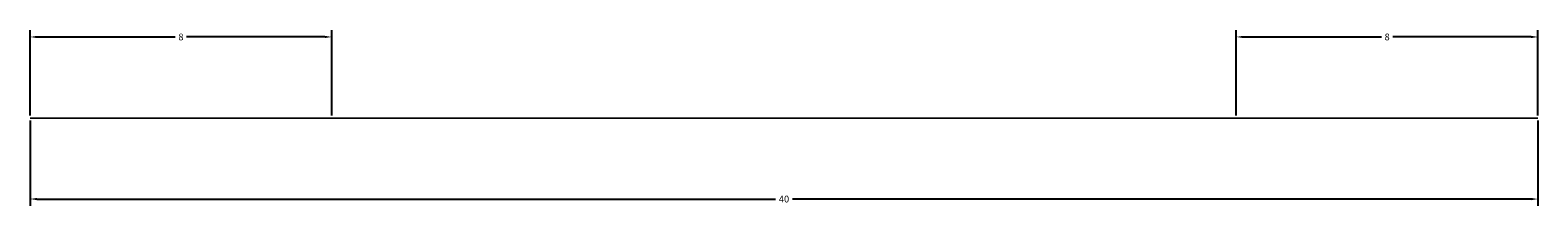
# Model space of a CAD drawing. Units: millimetres. Extents: x -4 to 2856, y -2 to 1373.
# Tile 2 of 3: x 2516 to 2556, y -2 to 2. Entities that reach past the tile are written whole.
import ezdxf

# ---------------------------------------------------------------- set-up
doc = ezdxf.new("R2010")
doc.units = ezdxf.units.MM
doc.layers.add('M-CONS', color=8, linetype='Continuous', lineweight=18)
doc.layers.add('M-DIMS', color=2, linetype='Continuous', lineweight=18)
doc.styles.get("Standard").update_dxf_attribs({"font": 'arial.ttf'})
doc.dimstyles.get("Standard").update_dxf_attribs({"dimtxt": 0.18, "dimasz": 0.18, "dimexe": 0.18, "dimexo": 0.0625, "dimgap": 0.09, "dimtad": 0, "dimtih": 1, "dimtoh": 1, "dimdec": 4, "dimzin": 0, "dimdsep": 46, "dimtxsty": 'Standard', "dimcen": 0.09, "dimadec": 0, "dimazin": 0, "dimtfac": 1, "dimtdec": 4, "dimtofl": 0, "dimtmove": 0, "dimatfit": 3, "dimfxl": 1, "dimtolj": 1, "dimtzin": 0, "dimarcsym": 0})

# ---------------------------------------------------------------- blocks, each defined once
blk = doc.blocks.new('*D7')
at = {"layer": 'Defpoints', "color": 0, "transparency": 16777216}
for p in [(2515.809, 0), (2555.809, 0), (2555.809, -2.15)]:
    blk.add_point(p, dxfattribs=at)
at = {"layer": 'M-DIMS', "color": 0, "lineweight": -2, "transparency": 16777216}
for p, q in [((2515.809, -0.062), (2515.809, -2.33)), ((2555.809, -0.062), (2555.809, -2.33)), ((2515.989, -2.15), (2535.586, -2.15)), ((2555.629, -2.15), (2536.031, -2.15))]:
    blk.add_line(p, q, dxfattribs=at)
at = {"layer": 'M-DIMS', "color": 0, "transparency": 16777216}
for points in [[(2515.989, -2.12), (2515.989, -2.18), (2515.809, -2.15)], [(2555.629, -2.12), (2555.629, -2.18), (2555.809, -2.15)]]:
    blk.add_solid(points, dxfattribs=at)
at = {"layer": 'M-DIMS', "color": 0, "transparency": 16777216, "insert": (2535.809, -2.15), "char_height": 0.18, "attachment_point": 5}
blk.add_mtext('\\A1;40', dxfattribs=at)
blk = doc.blocks.new('*D8')
at = {"layer": 'Defpoints', "color": 0, "transparency": 16777216}
for p in [(2523.809, 2.15), (2515.809, 0), (2523.809, 0)]:
    blk.add_point(p, dxfattribs=at)
at = {"layer": 'M-DIMS', "color": 0, "lineweight": -2, "transparency": 16777216}
for p, q in [((2515.809, 0.062), (2515.809, 2.33)), ((2515.989, 2.15), (2519.659, 2.15)), ((2523.629, 2.15), (2519.958, 2.15)), ((2523.809, 0.062), (2523.809, 2.33))]:
    blk.add_line(p, q, dxfattribs=at)
at = {"layer": 'M-DIMS', "color": 0, "transparency": 16777216}
for points in [[(2515.989, 2.18), (2515.989, 2.12), (2515.809, 2.15)], [(2523.629, 2.18), (2523.629, 2.12), (2523.809, 2.15)]]:
    blk.add_solid(points, dxfattribs=at)
at = {"layer": 'M-DIMS', "color": 0, "transparency": 16777216, "insert": (2519.809, 2.15), "char_height": 0.18, "attachment_point": 5}
blk.add_mtext('\\A1;8', dxfattribs=at)
blk = doc.blocks.new('*D9')
at = {"layer": 'Defpoints', "color": 0, "transparency": 16777216}
for p in [(2555.809, 2.15), (2547.809, 0), (2555.809, 0)]:
    blk.add_point(p, dxfattribs=at)
at = {"layer": 'M-DIMS', "color": 0, "lineweight": -2, "transparency": 16777216}
for p, q in [((2547.809, 0.062), (2547.809, 2.33)), ((2547.989, 2.15), (2551.659, 2.15)), ((2555.629, 2.15), (2551.958, 2.15)), ((2555.809, 0.062), (2555.809, 2.33))]:
    blk.add_line(p, q, dxfattribs=at)
at = {"layer": 'M-DIMS', "color": 0, "transparency": 16777216}
for points in [[(2547.989, 2.18), (2547.989, 2.12), (2547.809, 2.15)], [(2555.629, 2.18), (2555.629, 2.12), (2555.809, 2.15)]]:
    blk.add_solid(points, dxfattribs=at)
at = {"layer": 'M-DIMS', "color": 0, "transparency": 16777216, "insert": (2551.809, 2.15), "char_height": 0.18, "attachment_point": 5}
blk.add_mtext('\\A1;8', dxfattribs=at)

msp = doc.modelspace()

# ---------------------------------------------------------------- linework, layer by layer
at = {"layer": 'M-CONS', "extrusion": (0, -1, 0)}
msp.add_lwpolyline([(2555.809, 47.479), (2555.809, 19.479), (2547.809, 19.479), (2523.809, 19.479), (2515.809, 19.479), (2515.809, 47.479), (2523.809, 47.479, 1), (2547.809, 47.479)], format="xyb", close=True, dxfattribs=at)

# ---------------------------------------------------------------- dimensions: what is measured, and where the dimension line sits
at = {"layer": 'M-DIMS'}
for base, p1, p2, picture, middle in [((2523.809, 2.15), (2515.809, 0), (2523.809, 0), '*D8', (2519.809, 2.15)), ((2555.809, 2.15), (2547.809, 0), (2555.809, 0), '*D9', (2551.809, 2.15)), ((2555.809, -2.15), (2515.809, 0), (2555.809, 0), '*D7', (2535.809, -2.15))]:
    dim = msp.add_linear_dim(base=base, p1=p1, p2=p2, dimstyle='Standard', override={"dimdec": 0, "dimlfac": 1, "dimrnd": 0, "dimzin": 0, "dimdsep": 46, "dimlunit": 2}, dxfattribs=at)
    dim.commit()
    dim.dimension.update_dxf_attribs({"geometry": picture, "text_midpoint": middle})

doc.saveas('drawing.dxf')
